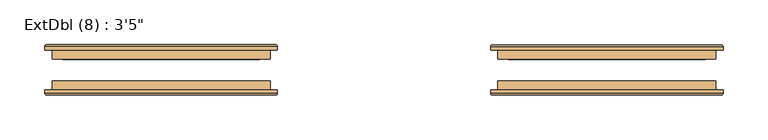
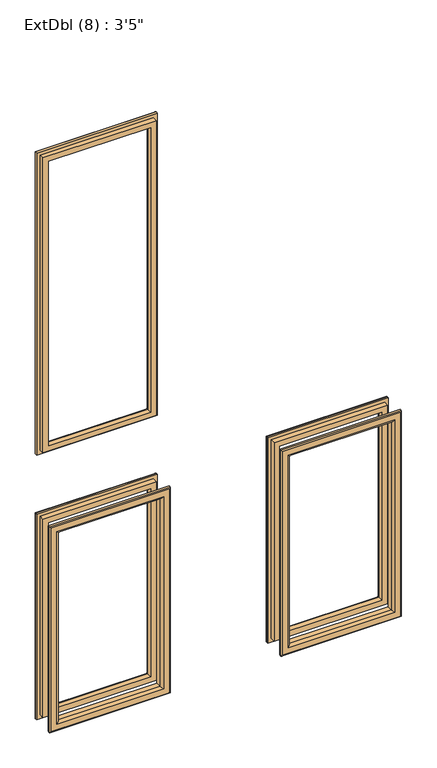
"""IFC4 building model written with IfcOpenShell, lengths in millimetres: door geometry."""

from ifc_helpers import new_model, si_unit, frame, origin, place, context, project, spatial, ellipse_curve, source, transform, mapped, element, save
from ifc_brep_helpers import plane_surface, cylinder_surface, advanced_brep


def door_f6085f53(model_context):
    return source(origin(), model_context, "Body", "AdvancedBrep", [
        advanced_brep(
        [(-377.2, 8.3, 950.5), (-377.2, 4.3, 950.5), (-377.2, 4.3, 1635.3), (-377.2, 8.3, 1635.3), (-375.2, 10.3, 952.5), (-375.2, 10.3, 1633.3), (-357.2, 5.3, 970.5), (-362.2, 10.3, 965.5), (-362.2, 10.3, 1620.3), (-357.2, 5.3, 1615.3), (-357.2, -5.7, 970.5), (-357.2, -5.7, 1615.3), (-369.2, 4.3, 958.5), (-369.2, -5.7, 958.5), (-369.2, -5.7, 1627.3), (-369.2, 4.3, 1627.3), (-118.5, 4.3, 1635.3), (-118.5, 8.3, 1635.3), (-120.5, 10.3, 1633.3), (-133.5, 10.3, 1620.3), (-138.5, 5.3, 1615.3), (-138.5, -5.7, 1615.3), (-126.5, -5.7, 1627.3), (-126.5, 4.3, 1627.3), (-118.5, 4.3, 950.5), (-118.5, 8.3, 950.5), (-120.5, 10.3, 952.5), (-133.5, 10.3, 965.5), (-138.5, 5.3, 970.5), (-138.5, -5.7, 970.5), (-126.5, -5.7, 958.5), (-126.5, 4.3, 958.5)],
        [
            (0, 1),
            (1, 2),
            (2, 3),
            (3, 0),
            (4, 0, ellipse_curve(frame((-375.2, 8.3, 952.5), z_axis=(-0.7071067811865472, 0.0, 0.7071067811865477), x_axis=(-0.7071067811865477, 0.0, -0.7071067811865475)), 2.8284271, 2.0)),
            (3, 5, ellipse_curve(frame((-375.2, 8.3, 1633.3), z_axis=(-0.7071067811865475, 0.0, -0.7071067811865475), x_axis=(0.7071067811865474, 0.0, -0.7071067811865476)), 2.8284271, 2.0)),
            (5, 4),
            (6, 7, ellipse_curve(frame((-362.2, 5.3, 965.5), z_axis=(-0.7071067811865472, 0.0, 0.7071067811865477), x_axis=(-0.7071067811865477, 0.0, -0.7071067811865475)), 7.0710678, 5.0)),
            (7, 8),
            (8, 9, ellipse_curve(frame((-362.2, 5.3, 1620.3), z_axis=(-0.7071067811865475, 0.0, -0.7071067811865475), x_axis=(0.7071067811865474, 0.0, -0.7071067811865476)), 7.0710678, 5.0)),
            (9, 6),
            (10, 6),
            (9, 11),
            (11, 10),
            (12, 13),
            (13, 14),
            (14, 15),
            (15, 12),
            (2, 16),
            (16, 17),
            (17, 3),
            (17, 18, ellipse_curve(frame((-120.5, 8.3, 1633.3), z_axis=(-0.7071067811865475, 0.0, 0.7071067811865476), x_axis=(-0.7071067811865476, 0.0, -0.7071067811865475)), 2.8284271, 2.0)),
            (18, 5),
            (8, 19),
            (19, 20, ellipse_curve(frame((-133.5, 5.3, 1620.3), z_axis=(-0.7071067811865475, 0.0, 0.7071067811865476), x_axis=(-0.7071067811865476, 0.0, -0.7071067811865475)), 7.0710678, 5.0)),
            (20, 9),
            (20, 21),
            (21, 11),
            (14, 22),
            (22, 23),
            (23, 15),
            (16, 24),
            (24, 25),
            (25, 17),
            (25, 26, ellipse_curve(frame((-120.5, 8.3, 952.5), z_axis=(0.7071067811865478, 0.0, 0.7071067811865472), x_axis=(-0.7071067811865472, 0.0, 0.7071067811865478)), 2.8284271, 2.0)),
            (26, 18),
            (19, 27),
            (27, 28, ellipse_curve(frame((-133.5, 5.3, 965.5), z_axis=(0.7071067811865478, 0.0, 0.7071067811865472), x_axis=(-0.7071067811865472, 0.0, 0.7071067811865478)), 7.0710678, 5.0)),
            (28, 20),
            (28, 29),
            (29, 21),
            (22, 30),
            (30, 31),
            (31, 23),
            (24, 1),
            (0, 25),
            (4, 26),
            (7, 27),
            (6, 28),
            (10, 29),
            (13, 30),
            (12, 31),
        ],
        [
            plane_surface(frame((-377.2, 4.3, 950.5), z_axis=(-1.0, 0.0, 0.0), x_axis=(0.0, 0.0, 1.0))),
            cylinder_surface(frame((-375.2, 8.3, 958.5), z_axis=(0.0, 0.0, -1.0), x_axis=(-1.0, 0.0, 0.0)), 2.0),
            cylinder_surface(frame((-362.2, 5.3, 958.5), z_axis=(0.0, 0.0, -1.0), x_axis=(-1.0, 0.0, 0.0)), 5.0),
            plane_surface(frame((-357.2, 5.3, 970.5), z_axis=(1.0, 0.0, 0.0), x_axis=(0.0, 0.0, 1.0))),
            plane_surface(frame((-369.2, -5.7, 958.5), z_axis=(-1.0, 0.0, 0.0), x_axis=(0.0, 0.0, 1.0))),
            plane_surface(frame((-377.2, 4.3, 1635.3), z_axis=(0.0, 0.0, 1.0), x_axis=(1.0, 0.0, 0.0))),
            cylinder_surface(frame((-369.2, 8.3, 1633.3), z_axis=(-1.0, 0.0, 0.0), x_axis=(0.0, 0.0, 1.0)), 2.0),
            cylinder_surface(frame((-369.2, 5.3, 1620.3), z_axis=(-1.0, 0.0, 0.0), x_axis=(0.0, 0.0, 1.0)), 5.0),
            plane_surface(frame((-357.2, 5.3, 1615.3), z_axis=(0.0, 0.0, -1.0), x_axis=(1.0, 0.0, 0.0))),
            plane_surface(frame((-369.2, -5.7, 1627.3), z_axis=(0.0, 0.0, 1.0), x_axis=(1.0, 0.0, 0.0))),
            plane_surface(frame((-118.5, 4.3, 1635.3), z_axis=(1.0, 0.0, 0.0), x_axis=(0.0, 0.0, -1.0))),
            cylinder_surface(frame((-120.5, 8.3, 1627.3), z_axis=(0.0, 0.0, 1.0), x_axis=(1.0, 0.0, 0.0)), 2.0),
            cylinder_surface(frame((-133.5, 5.3, 1627.3), z_axis=(0.0, 0.0, 1.0), x_axis=(1.0, 0.0, 0.0)), 5.0),
            plane_surface(frame((-138.5, 5.3, 1615.3), z_axis=(-1.0, 0.0, 0.0), x_axis=(0.0, 0.0, -1.0))),
            plane_surface(frame((-126.5, -5.7, 1627.3), z_axis=(1.0, 0.0, 0.0), x_axis=(0.0, 0.0, -1.0))),
            plane_surface(frame((-118.5, 4.3, 950.5), z_axis=(0.0, 0.0, -1.0), x_axis=(-1.0, 0.0, 0.0))),
            cylinder_surface(frame((-126.5, 8.3, 952.5), z_axis=(1.0, 0.0, 0.0), x_axis=(0.0, 0.0, -1.0)), 2.0),
            plane_surface(frame((-120.5, 10.3, 952.5), z_axis=(0.0, 1.0, 0.0), x_axis=(-1.0, 0.0, 0.0))),
            cylinder_surface(frame((-126.5, 5.3, 965.5), z_axis=(1.0, 0.0, 0.0), x_axis=(0.0, 0.0, -1.0)), 5.0),
            plane_surface(frame((-138.5, 5.3, 970.5), z_axis=(0.0, 0.0, 1.0), x_axis=(-1.0, 0.0, 0.0))),
            plane_surface(frame((-138.5, -5.7, 970.5), z_axis=(0.0, -1.0, 0.0), x_axis=(-1.0, 0.0, 0.0))),
            plane_surface(frame((-126.5, -5.7, 958.5), z_axis=(0.0, 0.0, -1.0), x_axis=(-1.0, 0.0, 0.0))),
            plane_surface(frame((-126.5, 4.3, 958.5), z_axis=(0.0, -1.0, 0.0), x_axis=(-1.0, 0.0, 0.0))),
        ],
        [
            (0, [[1, 2, 3, 4]]),
            (1, [[5, -4, 6, 7]]),
            (2, [[8, 9, 10, 11]]),
            (3, [[12, -11, 13, 14]]),
            (4, [[15, 16, 17, 18]]),
            (5, [[-3, 19, 20, 21]]),
            (6, [[-6, -21, 22, 23]]),
            (7, [[-10, 24, 25, 26]]),
            (8, [[-13, -26, 27, 28]]),
            (9, [[-17, 29, 30, 31]]),
            (10, [[-20, 32, 33, 34]]),
            (11, [[-22, -34, 35, 36]]),
            (12, [[-25, 37, 38, 39]]),
            (13, [[-27, -39, 40, 41]]),
            (14, [[-30, 42, 43, 44]]),
            (15, [[-33, 45, -1, 46]]),
            (16, [[-35, -46, -5, 47]]),
            (17, [[-23, -36, -47, -7], [48, -37, -24, -9]]),
            (18, [[-38, -48, -8, 49]]),
            (19, [[-40, -49, -12, 50]]),
            (20, [[51, -42, -29, -16], [-28, -41, -50, -14]]),
            (21, [[-43, -51, -15, 52]]),
            (22, [[-45, -32, -19, -2], [-31, -44, -52, -18]]),
        ],
    ),
        advanced_brep(
        [(126.5, -5.7, 808.5), (126.5, 4.3, 808.5), (126.5, 4.3, 358.5), (126.5, -5.7, 358.5), (138.5, 5.3, 796.5), (138.5, -5.7, 796.5), (138.5, -5.7, 370.5), (138.5, 5.3, 370.5), (133.5, 10.3, 801.5), (133.5, 10.3, 365.5), (118.5, 8.3, 816.5), (120.5, 10.3, 814.5), (120.5, 10.3, 352.5), (118.5, 8.3, 350.5), (118.5, 4.3, 816.5), (118.5, 4.3, 350.5), (369.2, 4.3, 358.5), (369.2, -5.7, 358.5), (357.2, -5.7, 370.5), (357.2, 5.3, 370.5), (362.2, 10.3, 365.5), (375.2, 10.3, 352.5), (377.2, 8.3, 350.5), (377.2, 4.3, 350.5), (369.2, 4.3, 808.5), (369.2, -5.7, 808.5), (357.2, -5.7, 796.5), (357.2, 5.3, 796.5), (362.2, 10.3, 801.5), (375.2, 10.3, 814.5), (377.2, 8.3, 816.5), (377.2, 4.3, 816.5)],
        [
            (0, 1),
            (1, 2),
            (2, 3),
            (3, 0),
            (4, 5),
            (5, 6),
            (6, 7),
            (7, 4),
            (8, 4, ellipse_curve(frame((133.5, 5.3, 801.5), z_axis=(-0.7071067811865475, 0.0, -0.7071067811865475), x_axis=(-0.7071067811865474, 0.0, 0.7071067811865476)), 7.0710678, 5.0)),
            (7, 9, ellipse_curve(frame((133.5, 5.3, 365.5), z_axis=(-0.7071067811865475, 0.0, 0.7071067811865475), x_axis=(0.7071067811865474, 0.0, 0.7071067811865476)), 7.0710678, 5.0)),
            (9, 8),
            (10, 11, ellipse_curve(frame((120.5, 8.3, 814.5), z_axis=(-0.7071067811865475, 0.0, -0.7071067811865475), x_axis=(-0.7071067811865474, 0.0, 0.7071067811865476)), 2.8284271, 2.0)),
            (11, 12),
            (12, 13, ellipse_curve(frame((120.5, 8.3, 352.5), z_axis=(-0.7071067811865475, 0.0, 0.7071067811865475), x_axis=(0.7071067811865474, 0.0, 0.7071067811865476)), 2.8284271, 2.0)),
            (13, 10),
            (14, 10),
            (13, 15),
            (15, 14),
            (2, 16),
            (16, 17),
            (17, 3),
            (6, 18),
            (18, 19),
            (19, 7),
            (19, 20, ellipse_curve(frame((362.2, 5.3, 365.5), z_axis=(-0.7071067811865476, 0.0, -0.7071067811865475), x_axis=(-0.7071067811865475, 0.0, 0.7071067811865476)), 7.0710678, 5.0)),
            (20, 9),
            (12, 21),
            (21, 22, ellipse_curve(frame((375.2, 8.3, 352.5), z_axis=(-0.7071067811865476, 0.0, -0.7071067811865475), x_axis=(-0.7071067811865475, 0.0, 0.7071067811865476)), 2.8284271, 2.0)),
            (22, 13),
            (22, 23),
            (23, 15),
            (16, 24),
            (24, 25),
            (25, 17),
            (18, 26),
            (26, 27),
            (27, 19),
            (27, 28, ellipse_curve(frame((362.2, 5.3, 801.5), z_axis=(0.7071067811865475, 0.0, -0.7071067811865476), x_axis=(-0.7071067811865476, 0.0, -0.7071067811865475)), 7.0710678, 5.0)),
            (28, 20),
            (21, 29),
            (29, 30, ellipse_curve(frame((375.2, 8.3, 814.5), z_axis=(0.7071067811865475, 0.0, -0.7071067811865476), x_axis=(-0.7071067811865476, 0.0, -0.7071067811865475)), 2.8284271, 2.0)),
            (30, 22),
            (30, 31),
            (31, 23),
            (31, 14),
            (1, 24),
            (0, 25),
            (5, 26),
            (4, 27),
            (8, 28),
            (11, 29),
            (10, 30),
        ],
        [
            plane_surface(frame((126.5, 4.3, 808.5), z_axis=(-1.0, 0.0, 0.0), x_axis=(0.0, 0.0, -1.0))),
            plane_surface(frame((138.5, -5.7, 796.5), z_axis=(1.0, 0.0, 0.0), x_axis=(0.0, 0.0, -1.0))),
            cylinder_surface(frame((133.5, 5.3, 808.5), z_axis=(0.0, 0.0, 1.0), x_axis=(-1.0, 0.0, 0.0)), 5.0),
            cylinder_surface(frame((120.5, 8.3, 808.5), z_axis=(0.0, 0.0, 1.0), x_axis=(-1.0, 0.0, 0.0)), 2.0),
            plane_surface(frame((118.5, 8.3, 816.5), z_axis=(-1.0, 0.0, 0.0), x_axis=(0.0, 0.0, -1.0))),
            plane_surface(frame((126.5, 4.3, 358.5), z_axis=(0.0, 0.0, -1.0), x_axis=(1.0, 0.0, 0.0))),
            plane_surface(frame((138.5, -5.7, 370.5), z_axis=(0.0, 0.0, 1.0), x_axis=(1.0, 0.0, 0.0))),
            cylinder_surface(frame((126.5, 5.3, 365.5), z_axis=(-1.0, 0.0, 0.0), x_axis=(0.0, 0.0, -1.0)), 5.0),
            cylinder_surface(frame((126.5, 8.3, 352.5), z_axis=(-1.0, 0.0, 0.0), x_axis=(0.0, 0.0, -1.0)), 2.0),
            plane_surface(frame((118.5, 8.3, 350.5), z_axis=(0.0, 0.0, -1.0), x_axis=(1.0, 0.0, 0.0))),
            plane_surface(frame((369.2, 4.3, 358.5), z_axis=(1.0, 0.0, 0.0), x_axis=(0.0, 0.0, 1.0))),
            plane_surface(frame((357.2, -5.7, 370.5), z_axis=(-1.0, 0.0, 0.0), x_axis=(0.0, 0.0, 1.0))),
            cylinder_surface(frame((362.2, 5.3, 358.5), z_axis=(0.0, 0.0, -1.0), x_axis=(1.0, 0.0, 0.0)), 5.0),
            cylinder_surface(frame((375.2, 8.3, 358.5), z_axis=(0.0, 0.0, -1.0), x_axis=(1.0, 0.0, 0.0)), 2.0),
            plane_surface(frame((377.2, 8.3, 350.5), z_axis=(1.0, 0.0, 0.0), x_axis=(0.0, 0.0, 1.0))),
            plane_surface(frame((377.2, 4.3, 816.5), z_axis=(0.0, -1.0, 0.0), x_axis=(-1.0, 0.0, 0.0))),
            plane_surface(frame((369.2, 4.3, 808.5), z_axis=(0.0, 0.0, 1.0), x_axis=(-1.0, 0.0, 0.0))),
            plane_surface(frame((369.2, -5.7, 808.5), z_axis=(0.0, -1.0, 0.0), x_axis=(-1.0, 0.0, 0.0))),
            plane_surface(frame((357.2, -5.7, 796.5), z_axis=(0.0, 0.0, -1.0), x_axis=(-1.0, 0.0, 0.0))),
            cylinder_surface(frame((369.2, 5.3, 801.5), z_axis=(1.0, 0.0, 0.0), x_axis=(0.0, 0.0, 1.0)), 5.0),
            plane_surface(frame((362.2, 10.3, 801.5), z_axis=(0.0, 1.0, 0.0), x_axis=(-1.0, 0.0, 0.0))),
            cylinder_surface(frame((369.2, 8.3, 814.5), z_axis=(1.0, 0.0, 0.0), x_axis=(0.0, 0.0, 1.0)), 2.0),
            plane_surface(frame((377.2, 8.3, 816.5), z_axis=(0.0, 0.0, 1.0), x_axis=(-1.0, 0.0, 0.0))),
        ],
        [
            (0, [[1, 2, 3, 4]]),
            (1, [[5, 6, 7, 8]]),
            (2, [[9, -8, 10, 11]]),
            (3, [[12, 13, 14, 15]]),
            (4, [[16, -15, 17, 18]]),
            (5, [[-3, 19, 20, 21]]),
            (6, [[-7, 22, 23, 24]]),
            (7, [[-10, -24, 25, 26]]),
            (8, [[-14, 27, 28, 29]]),
            (9, [[-17, -29, 30, 31]]),
            (10, [[-20, 32, 33, 34]]),
            (11, [[-23, 35, 36, 37]]),
            (12, [[-25, -37, 38, 39]]),
            (13, [[-28, 40, 41, 42]]),
            (14, [[-30, -42, 43, 44]]),
            (15, [[-31, -44, 45, -18], [46, -32, -19, -2]]),
            (16, [[-33, -46, -1, 47]]),
            (17, [[-21, -34, -47, -4], [48, -35, -22, -6]]),
            (18, [[-36, -48, -5, 49]]),
            (19, [[-38, -49, -9, 50]]),
            (20, [[51, -40, -27, -13], [-26, -39, -50, -11]]),
            (21, [[-41, -51, -12, 52]]),
            (22, [[-43, -52, -16, -45]]),
        ],
    ),
        advanced_brep(
        [(369.2, -29.7, 808.5), (369.2, -39.7, 808.5), (369.2, -39.7, 358.5), (369.2, -29.7, 358.5), (357.2, -40.7, 796.5), (357.2, -29.7, 796.5), (357.2, -29.7, 370.5), (357.2, -40.7, 370.5), (362.2, -45.7, 801.5), (362.2, -45.7, 365.5), (377.2, -43.7, 816.5), (375.2, -45.7, 814.5), (375.2, -45.7, 352.5), (377.2, -43.7, 350.5), (377.2, -39.7, 816.5), (377.2, -39.7, 350.5), (126.5, -39.7, 358.5), (126.5, -29.7, 358.5), (138.5, -29.7, 370.5), (138.5, -40.7, 370.5), (133.5, -45.7, 365.5), (120.5, -45.7, 352.5), (118.5, -43.7, 350.5), (118.5, -39.7, 350.5), (126.5, -39.7, 808.5), (126.5, -29.7, 808.5), (138.5, -29.7, 796.5), (138.5, -40.7, 796.5), (133.5, -45.7, 801.5), (120.5, -45.7, 814.5), (118.5, -43.7, 816.5), (118.5, -39.7, 816.5)],
        [
            (0, 1),
            (1, 2),
            (2, 3),
            (3, 0),
            (4, 5),
            (5, 6),
            (6, 7),
            (7, 4),
            (8, 4, ellipse_curve(frame((362.2, -40.7, 801.5), z_axis=(0.7071067811865519, 0.0, -0.707106781186543), x_axis=(0.7071067811865429, 0.0, 0.7071067811865521)), 7.0710678, 5.0)),
            (7, 9, ellipse_curve(frame((362.2, -40.7, 365.5), z_axis=(0.7071067811865429, 0.0, 0.707106781186552), x_axis=(-0.7071067811865519, 0.0, 0.707106781186543)), 7.0710678, 5.0)),
            (9, 8),
            (10, 11, ellipse_curve(frame((375.2, -43.7, 814.5), z_axis=(0.7071067811865519, 0.0, -0.707106781186543), x_axis=(0.7071067811865429, 0.0, 0.7071067811865521)), 2.8284271, 2.0)),
            (11, 12),
            (12, 13, ellipse_curve(frame((375.2, -43.7, 352.5), z_axis=(0.7071067811865429, 0.0, 0.707106781186552), x_axis=(-0.7071067811865519, 0.0, 0.707106781186543)), 2.8284271, 2.0)),
            (13, 10),
            (14, 10),
            (13, 15),
            (15, 14),
            (2, 16),
            (16, 17),
            (17, 3),
            (6, 18),
            (18, 19),
            (19, 7),
            (19, 20, ellipse_curve(frame((133.5, -40.7, 365.5), z_axis=(0.707106781186552, 0.0, -0.7071067811865429), x_axis=(0.707106781186543, 0.0, 0.7071067811865519)), 7.0710678, 5.0)),
            (20, 9),
            (12, 21),
            (21, 22, ellipse_curve(frame((120.5, -43.7, 352.5), z_axis=(0.707106781186552, 0.0, -0.7071067811865429), x_axis=(0.707106781186543, 0.0, 0.7071067811865519)), 2.8284271, 2.0)),
            (22, 13),
            (22, 23),
            (23, 15),
            (16, 24),
            (24, 25),
            (25, 17),
            (18, 26),
            (26, 27),
            (27, 19),
            (27, 28, ellipse_curve(frame((133.5, -40.7, 801.5), z_axis=(-0.7071067811865431, 0.0, -0.707106781186552), x_axis=(0.7071067811865521, 0.0, -0.7071067811865429)), 7.0710678, 5.0)),
            (28, 20),
            (21, 29),
            (29, 30, ellipse_curve(frame((120.5, -43.7, 814.5), z_axis=(-0.7071067811865431, 0.0, -0.707106781186552), x_axis=(0.7071067811865521, 0.0, -0.7071067811865429)), 2.8284271, 2.0)),
            (30, 22),
            (30, 31),
            (31, 23),
            (31, 14),
            (1, 24),
            (0, 25),
            (5, 26),
            (4, 27),
            (8, 28),
            (11, 29),
            (10, 30),
        ],
        [
            plane_surface(frame((369.2, -39.7, 808.5), z_axis=(1.0, 0.0, 0.0), x_axis=(0.0, 0.0, -1.0))),
            plane_surface(frame((357.2, -29.7, 796.5), z_axis=(-1.0, 0.0, 0.0), x_axis=(0.0, 0.0, -1.0))),
            cylinder_surface(frame((362.2, -40.7, 808.5), z_axis=(0.0, 0.0, 1.0), x_axis=(1.0, 0.0, 0.0)), 5.0),
            cylinder_surface(frame((375.2, -43.7, 808.5), z_axis=(0.0, 0.0, 1.0), x_axis=(1.0, 0.0, 0.0)), 2.0),
            plane_surface(frame((377.2, -43.7, 816.5), z_axis=(1.0, 0.0, 0.0), x_axis=(0.0, 0.0, -1.0))),
            plane_surface(frame((369.2, -39.7, 358.5), z_axis=(0.0, 0.0, -1.0), x_axis=(-1.0, 0.0, 0.0))),
            plane_surface(frame((357.2, -29.7, 370.5), z_axis=(0.0, 0.0, 1.0), x_axis=(-1.0, 0.0, 0.0))),
            cylinder_surface(frame((369.2, -40.7, 365.5), z_axis=(1.0, 0.0, 0.0), x_axis=(0.0, 0.0, -1.0)), 5.0),
            cylinder_surface(frame((369.2, -43.7, 352.5), z_axis=(1.0, 0.0, 0.0), x_axis=(0.0, 0.0, -1.0)), 2.0),
            plane_surface(frame((377.2, -43.7, 350.5), z_axis=(0.0, 0.0, -1.0), x_axis=(-1.0, 0.0, 0.0))),
            plane_surface(frame((126.5, -39.7, 358.5), z_axis=(-1.0, 0.0, 0.0), x_axis=(0.0, 0.0, 1.0))),
            plane_surface(frame((138.5, -29.7, 370.5), z_axis=(1.0, 0.0, 0.0), x_axis=(0.0, 0.0, 1.0))),
            cylinder_surface(frame((133.5, -40.7, 358.5), z_axis=(0.0, 0.0, -1.0), x_axis=(-1.0, 0.0, 0.0)), 5.0),
            cylinder_surface(frame((120.5, -43.7, 358.5), z_axis=(0.0, 0.0, -1.0), x_axis=(-1.0, 0.0, 0.0)), 2.0),
            plane_surface(frame((118.5, -43.7, 350.5), z_axis=(-1.0, 0.0, 0.0), x_axis=(0.0, 0.0, 1.0))),
            plane_surface(frame((118.5, -39.7, 816.5), z_axis=(0.0, 1.0, 0.0), x_axis=(1.0, 0.0, 0.0))),
            plane_surface(frame((126.5, -39.7, 808.5), z_axis=(0.0, 0.0, 1.0), x_axis=(1.0, 0.0, 0.0))),
            plane_surface(frame((126.5, -29.7, 808.5), z_axis=(0.0, 1.0, 0.0), x_axis=(1.0, 0.0, 0.0))),
            plane_surface(frame((138.5, -29.7, 796.5), z_axis=(0.0, 0.0, -1.0), x_axis=(1.0, 0.0, 0.0))),
            cylinder_surface(frame((126.5, -40.7, 801.5), z_axis=(-1.0, 0.0, 0.0), x_axis=(0.0, 0.0, 1.0)), 5.0),
            plane_surface(frame((133.5, -45.7, 801.5), z_axis=(0.0, -1.0, 0.0), x_axis=(1.0, 0.0, 0.0))),
            cylinder_surface(frame((126.5, -43.7, 814.5), z_axis=(-1.0, 0.0, 0.0), x_axis=(0.0, 0.0, 1.0)), 2.0),
            plane_surface(frame((118.5, -43.7, 816.5), z_axis=(0.0, 0.0, 1.0), x_axis=(1.0, 0.0, 0.0))),
        ],
        [
            (0, [[1, 2, 3, 4]]),
            (1, [[5, 6, 7, 8]]),
            (2, [[9, -8, 10, 11]]),
            (3, [[12, 13, 14, 15]]),
            (4, [[16, -15, 17, 18]]),
            (5, [[-3, 19, 20, 21]]),
            (6, [[-7, 22, 23, 24]]),
            (7, [[-10, -24, 25, 26]]),
            (8, [[-14, 27, 28, 29]]),
            (9, [[-17, -29, 30, 31]]),
            (10, [[-20, 32, 33, 34]]),
            (11, [[-23, 35, 36, 37]]),
            (12, [[-25, -37, 38, 39]]),
            (13, [[-28, 40, 41, 42]]),
            (14, [[-30, -42, 43, 44]]),
            (15, [[-31, -44, 45, -18], [46, -32, -19, -2]]),
            (16, [[-33, -46, -1, 47]]),
            (17, [[-21, -34, -47, -4], [48, -35, -22, -6]]),
            (18, [[-36, -48, -5, 49]]),
            (19, [[-38, -49, -9, 50]]),
            (20, [[51, -40, -27, -13], [-26, -39, -50, -11]]),
            (21, [[-41, -51, -12, 52]]),
            (22, [[-43, -52, -16, -45]]),
        ],
    ),
        advanced_brep(
        [(-369.2, -5.7, 808.5), (-369.2, 4.3, 808.5), (-369.2, 4.3, 358.5), (-369.2, -5.7, 358.5), (-357.2, 5.3, 796.5), (-357.2, -5.7, 796.5), (-357.2, -5.7, 370.5), (-357.2, 5.3, 370.5), (-362.2, 10.3, 801.5), (-362.2, 10.3, 365.5), (-377.2, 8.3, 816.5), (-375.2, 10.3, 814.5), (-375.2, 10.3, 352.5), (-377.2, 8.3, 350.5), (-377.2, 4.3, 816.5), (-377.2, 4.3, 350.5), (-126.5, 4.3, 358.5), (-126.5, -5.7, 358.5), (-138.5, -5.7, 370.5), (-138.5, 5.3, 370.5), (-133.5, 10.3, 365.5), (-120.5, 10.3, 352.5), (-118.5, 8.3, 350.5), (-118.5, 4.3, 350.5), (-126.5, 4.3, 808.5), (-126.5, -5.7, 808.5), (-138.5, -5.7, 796.5), (-138.5, 5.3, 796.5), (-133.5, 10.3, 801.5), (-120.5, 10.3, 814.5), (-118.5, 8.3, 816.5), (-118.5, 4.3, 816.5)],
        [
            (0, 1),
            (1, 2),
            (2, 3),
            (3, 0),
            (4, 5),
            (5, 6),
            (6, 7),
            (7, 4),
            (8, 4, ellipse_curve(frame((-362.2, 5.3, 801.5), z_axis=(-0.7071067811865478, 0.0, -0.7071067811865474), x_axis=(-0.7071067811865474, 0.0, 0.7071067811865476)), 7.0710678, 5.0)),
            (7, 9, ellipse_curve(frame((-362.2, 5.3, 365.5), z_axis=(-0.7071067811865475, 0.0, 0.7071067811865475), x_axis=(0.7071067811865474, 0.0, 0.7071067811865476)), 7.0710678, 5.0)),
            (9, 8),
            (10, 11, ellipse_curve(frame((-375.2, 8.3, 814.5), z_axis=(-0.7071067811865478, 0.0, -0.7071067811865474), x_axis=(-0.7071067811865474, 0.0, 0.7071067811865476)), 2.8284271, 2.0)),
            (11, 12),
            (12, 13, ellipse_curve(frame((-375.2, 8.3, 352.5), z_axis=(-0.7071067811865475, 0.0, 0.7071067811865475), x_axis=(0.7071067811865474, 0.0, 0.7071067811865476)), 2.8284271, 2.0)),
            (13, 10),
            (14, 10),
            (13, 15),
            (15, 14),
            (2, 16),
            (16, 17),
            (17, 3),
            (6, 18),
            (18, 19),
            (19, 7),
            (19, 20, ellipse_curve(frame((-133.5, 5.3, 365.5), z_axis=(-0.7071067811865475, 0.0, -0.7071067811865475), x_axis=(-0.7071067811865476, 0.0, 0.7071067811865474)), 7.0710678, 5.0)),
            (20, 9),
            (12, 21),
            (21, 22, ellipse_curve(frame((-120.5, 8.3, 352.5), z_axis=(-0.7071067811865475, 0.0, -0.7071067811865475), x_axis=(-0.7071067811865476, 0.0, 0.7071067811865474)), 2.8284271, 2.0)),
            (22, 13),
            (22, 23),
            (23, 15),
            (16, 24),
            (24, 25),
            (25, 17),
            (18, 26),
            (26, 27),
            (27, 19),
            (27, 28, ellipse_curve(frame((-133.5, 5.3, 801.5), z_axis=(0.7071067811865472, 0.0, -0.7071067811865477), x_axis=(-0.7071067811865477, 0.0, -0.7071067811865475)), 7.0710678, 5.0)),
            (28, 20),
            (21, 29),
            (29, 30, ellipse_curve(frame((-120.5, 8.3, 814.5), z_axis=(0.7071067811865472, 0.0, -0.7071067811865477), x_axis=(-0.7071067811865477, 0.0, -0.7071067811865475)), 2.8284271, 2.0)),
            (30, 22),
            (30, 31),
            (31, 23),
            (31, 14),
            (1, 24),
            (0, 25),
            (5, 26),
            (4, 27),
            (8, 28),
            (11, 29),
            (10, 30),
        ],
        [
            plane_surface(frame((-369.2, 4.3, 808.5), z_axis=(-1.0, 0.0, 0.0), x_axis=(0.0, 0.0, -1.0))),
            plane_surface(frame((-357.2, -5.7, 796.5), z_axis=(1.0, 0.0, 0.0), x_axis=(0.0, 0.0, -1.0))),
            cylinder_surface(frame((-362.2, 5.3, 808.5), z_axis=(0.0, 0.0, 1.0), x_axis=(-1.0, 0.0, 0.0)), 5.0),
            cylinder_surface(frame((-375.2, 8.3, 808.5), z_axis=(0.0, 0.0, 1.0), x_axis=(-1.0, 0.0, 0.0)), 2.0),
            plane_surface(frame((-377.2, 8.3, 816.5), z_axis=(-1.0, 0.0, 0.0), x_axis=(0.0, 0.0, -1.0))),
            plane_surface(frame((-369.2, 4.3, 358.5), z_axis=(0.0, 0.0, -1.0), x_axis=(1.0, 0.0, 0.0))),
            plane_surface(frame((-357.2, -5.7, 370.5), z_axis=(0.0, 0.0, 1.0), x_axis=(1.0, 0.0, 0.0))),
            cylinder_surface(frame((-369.2, 5.3, 365.5), z_axis=(-1.0, 0.0, 0.0), x_axis=(0.0, 0.0, -1.0)), 5.0),
            cylinder_surface(frame((-369.2, 8.3, 352.5), z_axis=(-1.0, 0.0, 0.0), x_axis=(0.0, 0.0, -1.0)), 2.0),
            plane_surface(frame((-377.2, 8.3, 350.5), z_axis=(0.0, 0.0, -1.0), x_axis=(1.0, 0.0, 0.0))),
            plane_surface(frame((-126.5, 4.3, 358.5), z_axis=(1.0, 0.0, 0.0), x_axis=(0.0, 0.0, 1.0))),
            plane_surface(frame((-138.5, -5.7, 370.5), z_axis=(-1.0, 0.0, 0.0), x_axis=(0.0, 0.0, 1.0))),
            cylinder_surface(frame((-133.5, 5.3, 358.5), z_axis=(0.0, 0.0, -1.0), x_axis=(1.0, 0.0, 0.0)), 5.0),
            cylinder_surface(frame((-120.5, 8.3, 358.5), z_axis=(0.0, 0.0, -1.0), x_axis=(1.0, 0.0, 0.0)), 2.0),
            plane_surface(frame((-118.5, 8.3, 350.5), z_axis=(1.0, 0.0, 0.0), x_axis=(0.0, 0.0, 1.0))),
            plane_surface(frame((-118.5, 4.3, 816.5), z_axis=(0.0, -1.0, 0.0), x_axis=(-1.0, 0.0, 0.0))),
            plane_surface(frame((-126.5, 4.3, 808.5), z_axis=(0.0, 0.0, 1.0), x_axis=(-1.0, 0.0, 0.0))),
            plane_surface(frame((-126.5, -5.7, 808.5), z_axis=(0.0, -1.0, 0.0), x_axis=(-1.0, 0.0, 0.0))),
            plane_surface(frame((-138.5, -5.7, 796.5), z_axis=(0.0, 0.0, -1.0), x_axis=(-1.0, 0.0, 0.0))),
            cylinder_surface(frame((-126.5, 5.3, 801.5), z_axis=(1.0, 0.0, 0.0), x_axis=(0.0, 0.0, 1.0)), 5.0),
            plane_surface(frame((-133.5, 10.3, 801.5), z_axis=(0.0, 1.0, 0.0), x_axis=(-1.0, 0.0, 0.0))),
            cylinder_surface(frame((-126.5, 8.3, 814.5), z_axis=(1.0, 0.0, 0.0), x_axis=(0.0, 0.0, 1.0)), 2.0),
            plane_surface(frame((-118.5, 8.3, 816.5), z_axis=(0.0, 0.0, 1.0), x_axis=(-1.0, 0.0, 0.0))),
        ],
        [
            (0, [[1, 2, 3, 4]]),
            (1, [[5, 6, 7, 8]]),
            (2, [[9, -8, 10, 11]]),
            (3, [[12, 13, 14, 15]]),
            (4, [[16, -15, 17, 18]]),
            (5, [[-3, 19, 20, 21]]),
            (6, [[-7, 22, 23, 24]]),
            (7, [[-10, -24, 25, 26]]),
            (8, [[-14, 27, 28, 29]]),
            (9, [[-17, -29, 30, 31]]),
            (10, [[-20, 32, 33, 34]]),
            (11, [[-23, 35, 36, 37]]),
            (12, [[-25, -37, 38, 39]]),
            (13, [[-28, 40, 41, 42]]),
            (14, [[-30, -42, 43, 44]]),
            (15, [[-31, -44, 45, -18], [46, -32, -19, -2]]),
            (16, [[-33, -46, -1, 47]]),
            (17, [[-21, -34, -47, -4], [48, -35, -22, -6]]),
            (18, [[-36, -48, -5, 49]]),
            (19, [[-38, -49, -9, 50]]),
            (20, [[51, -40, -27, -13], [-26, -39, -50, -11]]),
            (21, [[-41, -51, -12, 52]]),
            (22, [[-43, -52, -16, -45]]),
        ],
    ),
        advanced_brep(
        [(-126.5, -29.7, 808.5), (-126.5, -39.7, 808.5), (-126.5, -39.7, 358.5), (-126.5, -29.7, 358.5), (-138.5, -40.7, 796.5), (-138.5, -29.7, 796.5), (-138.5, -29.7, 370.5), (-138.5, -40.7, 370.5), (-133.5, -45.7, 801.5), (-133.5, -45.7, 365.5), (-118.5, -43.7, 816.5), (-120.5, -45.7, 814.5), (-120.5, -45.7, 352.5), (-118.5, -43.7, 350.5), (-118.5, -39.7, 816.5), (-118.5, -39.7, 350.5), (-369.2, -39.7, 358.5), (-369.2, -29.7, 358.5), (-357.2, -29.7, 370.5), (-357.2, -40.7, 370.5), (-362.2, -45.7, 365.5), (-375.2, -45.7, 352.5), (-377.2, -43.7, 350.5), (-377.2, -39.7, 350.5), (-369.2, -39.7, 808.5), (-369.2, -29.7, 808.5), (-357.2, -29.7, 796.5), (-357.2, -40.7, 796.5), (-362.2, -45.7, 801.5), (-375.2, -45.7, 814.5), (-377.2, -43.7, 816.5), (-377.2, -39.7, 816.5)],
        [
            (0, 1),
            (1, 2),
            (2, 3),
            (3, 0),
            (4, 5),
            (5, 6),
            (6, 7),
            (7, 4),
            (8, 4, ellipse_curve(frame((-133.5, -40.7, 801.5), z_axis=(0.7071067811865521, 0.0, -0.707106781186543), x_axis=(0.707106781186543, 0.0, 0.707106781186552)), 7.0710678, 5.0)),
            (7, 9, ellipse_curve(frame((-133.5, -40.7, 365.5), z_axis=(0.707106781186543, 0.0, 0.707106781186552), x_axis=(-0.707106781186552, 0.0, 0.707106781186543)), 7.0710678, 5.0)),
            (9, 8),
            (10, 11, ellipse_curve(frame((-120.5, -43.7, 814.5), z_axis=(0.7071067811865521, 0.0, -0.707106781186543), x_axis=(0.707106781186543, 0.0, 0.707106781186552)), 2.8284271, 2.0)),
            (11, 12),
            (12, 13, ellipse_curve(frame((-120.5, -43.7, 352.5), z_axis=(0.707106781186543, 0.0, 0.707106781186552), x_axis=(-0.707106781186552, 0.0, 0.707106781186543)), 2.8284271, 2.0)),
            (13, 10),
            (14, 10),
            (13, 15),
            (15, 14),
            (2, 16),
            (16, 17),
            (17, 3),
            (6, 18),
            (18, 19),
            (19, 7),
            (19, 20, ellipse_curve(frame((-362.2, -40.7, 365.5), z_axis=(0.707106781186552, 0.0, -0.7071067811865429), x_axis=(0.707106781186543, 0.0, 0.707106781186552)), 7.0710678, 5.0)),
            (20, 9),
            (12, 21),
            (21, 22, ellipse_curve(frame((-375.2, -43.7, 352.5), z_axis=(0.707106781186552, 0.0, -0.7071067811865429), x_axis=(0.707106781186543, 0.0, 0.707106781186552)), 2.8284271, 2.0)),
            (22, 13),
            (22, 23),
            (23, 15),
            (16, 24),
            (24, 25),
            (25, 17),
            (18, 26),
            (26, 27),
            (27, 19),
            (27, 28, ellipse_curve(frame((-362.2, -40.7, 801.5), z_axis=(-0.7071067811865428, 0.0, -0.7071067811865521), x_axis=(0.707106781186552, 0.0, -0.7071067811865429)), 7.0710678, 5.0)),
            (28, 20),
            (21, 29),
            (29, 30, ellipse_curve(frame((-375.2, -43.7, 814.5), z_axis=(-0.7071067811865428, 0.0, -0.7071067811865521), x_axis=(0.707106781186552, 0.0, -0.7071067811865429)), 2.8284271, 2.0)),
            (30, 22),
            (30, 31),
            (31, 23),
            (31, 14),
            (1, 24),
            (0, 25),
            (5, 26),
            (4, 27),
            (8, 28),
            (11, 29),
            (10, 30),
        ],
        [
            plane_surface(frame((-126.5, -39.7, 808.5), z_axis=(1.0, 0.0, 0.0), x_axis=(0.0, 0.0, -1.0))),
            plane_surface(frame((-138.5, -29.7, 796.5), z_axis=(-1.0, 0.0, 0.0), x_axis=(0.0, 0.0, -1.0))),
            cylinder_surface(frame((-133.5, -40.7, 808.5), z_axis=(0.0, 0.0, 1.0), x_axis=(1.0, 0.0, 0.0)), 5.0),
            cylinder_surface(frame((-120.5, -43.7, 808.5), z_axis=(0.0, 0.0, 1.0), x_axis=(1.0, 0.0, 0.0)), 2.0),
            plane_surface(frame((-118.5, -43.7, 816.5), z_axis=(1.0, 0.0, 0.0), x_axis=(0.0, 0.0, -1.0))),
            plane_surface(frame((-126.5, -39.7, 358.5), z_axis=(0.0, 0.0, -1.0), x_axis=(-1.0, 0.0, 0.0))),
            plane_surface(frame((-138.5, -29.7, 370.5), z_axis=(0.0, 0.0, 1.0), x_axis=(-1.0, 0.0, 0.0))),
            cylinder_surface(frame((-126.5, -40.7, 365.5), z_axis=(1.0, 0.0, 0.0), x_axis=(0.0, 0.0, -1.0)), 5.0),
            cylinder_surface(frame((-126.5, -43.7, 352.5), z_axis=(1.0, 0.0, 0.0), x_axis=(0.0, 0.0, -1.0)), 2.0),
            plane_surface(frame((-118.5, -43.7, 350.5), z_axis=(0.0, 0.0, -1.0), x_axis=(-1.0, 0.0, 0.0))),
            plane_surface(frame((-369.2, -39.7, 358.5), z_axis=(-1.0, 0.0, 0.0), x_axis=(0.0, 0.0, 1.0))),
            plane_surface(frame((-357.2, -29.7, 370.5), z_axis=(1.0, 0.0, 0.0), x_axis=(0.0, 0.0, 1.0))),
            cylinder_surface(frame((-362.2, -40.7, 358.5), z_axis=(0.0, 0.0, -1.0), x_axis=(-1.0, 0.0, 0.0)), 5.0),
            cylinder_surface(frame((-375.2, -43.7, 358.5), z_axis=(0.0, 0.0, -1.0), x_axis=(-1.0, 0.0, 0.0)), 2.0),
            plane_surface(frame((-377.2, -43.7, 350.5), z_axis=(-1.0, 0.0, 0.0), x_axis=(0.0, 0.0, 1.0))),
            plane_surface(frame((-377.2, -39.7, 816.5), z_axis=(0.0, 1.0, 0.0), x_axis=(1.0, 0.0, 0.0))),
            plane_surface(frame((-369.2, -39.7, 808.5), z_axis=(0.0, 0.0, 1.0), x_axis=(1.0, 0.0, 0.0))),
            plane_surface(frame((-369.2, -29.7, 808.5), z_axis=(0.0, 1.0, 0.0), x_axis=(1.0, 0.0, 0.0))),
            plane_surface(frame((-357.2, -29.7, 796.5), z_axis=(0.0, 0.0, -1.0), x_axis=(1.0, 0.0, 0.0))),
            cylinder_surface(frame((-369.2, -40.7, 801.5), z_axis=(-1.0, 0.0, 0.0), x_axis=(0.0, 0.0, 1.0)), 5.0),
            plane_surface(frame((-362.2, -45.7, 801.5), z_axis=(0.0, -1.0, 0.0), x_axis=(1.0, 0.0, 0.0))),
            cylinder_surface(frame((-369.2, -43.7, 814.5), z_axis=(-1.0, 0.0, 0.0), x_axis=(0.0, 0.0, 1.0)), 2.0),
            plane_surface(frame((-377.2, -43.7, 816.5), z_axis=(0.0, 0.0, 1.0), x_axis=(1.0, 0.0, 0.0))),
        ],
        [
            (0, [[1, 2, 3, 4]]),
            (1, [[5, 6, 7, 8]]),
            (2, [[9, -8, 10, 11]]),
            (3, [[12, 13, 14, 15]]),
            (4, [[16, -15, 17, 18]]),
            (5, [[-3, 19, 20, 21]]),
            (6, [[-7, 22, 23, 24]]),
            (7, [[-10, -24, 25, 26]]),
            (8, [[-14, 27, 28, 29]]),
            (9, [[-17, -29, 30, 31]]),
            (10, [[-20, 32, 33, 34]]),
            (11, [[-23, 35, 36, 37]]),
            (12, [[-25, -37, 38, 39]]),
            (13, [[-28, 40, 41, 42]]),
            (14, [[-30, -42, 43, 44]]),
            (15, [[-31, -44, 45, -18], [46, -32, -19, -2]]),
            (16, [[-33, -46, -1, 47]]),
            (17, [[-21, -34, -47, -4], [48, -35, -22, -6]]),
            (18, [[-36, -48, -5, 49]]),
            (19, [[-38, -49, -9, 50]]),
            (20, [[51, -40, -27, -13], [-26, -39, -50, -11]]),
            (21, [[-41, -51, -12, 52]]),
            (22, [[-43, -52, -16, -45]]),
        ],
    ),
    ])


if __name__ == "__main__":
    model = new_model("IFC4")
    model_context = context("Model", 3, world=origin())
    ifc_project = project(units=[si_unit("LENGTHUNIT", "METRE", prefix="MILLI")], contexts=[model_context])
    site = spatial("IfcSite", under=ifc_project)
    building = spatial("IfcBuilding", under=site)
    placement = place(None, origin())
    door_shape = door_f6085f53(model_context)
    element("IfcDoor", 1, ObjectType="ExtDbl (8) : 3'5\"", at=placement, inside=building, context=model_context, shape_type="MappedRepresentation", body=[
        mapped(door_shape, transform((0.0, 0.0, 0.0), x_axis=(1.0, 0.0, 0.0), y_axis=(0.0, 1.0, 0.0), z_axis=(0.0, 0.0, 1.0))),
    ])
    save(model, "model.ifc")

# Revit data of these elements
# Type "ExtDbl (8) : 3'5\""
#   Type Mark = "46"
#   Operation = "DoubleDoorSingleSwing"
#   Keynote = "L20"
#   Wrap Layers (Int) from Ext = 0' - 6.98819"
#   Wrap Layers (Ext) from Ext = 0' - 4.03543"
#   Top of Lock Rail = 2' - 11.43307"
#   Thickness = 0' - 1.73228"
#   Stile Shutting = 0' - 4.92126"
#   Stile - Top Rail = 0' - 5.90551"
#   Stile - Lock Rail = 0' - 5.90551"
#   Stile - Hanging = 0' - 3.93701"
#   Stile - Bottom Rail = 0' - 11.81102"
#   Rough Width = 3' - 5"
#   Rough Height = 6' - 0"
#   O/A Frame Width = 0' - 2.51969"
#   Handle Z Distance = 3' - 1.40157"
#   Glazing Thickness = 0' - 0.94488"
#   FrameWidth = 0' - 1.65354"
#   FrameOffset - External = 0' - 2.55906"
#   FrameDepth = 0' - 3.50394"
#   Door Panel Width = 1' - 6.41339"
#   Door Panel Thickness = 0' - 1.73228"
#   Door Panel Height = 5' - 7.66929"
#   Cill Thickness = 0' - 2.14567"
#   Cill Projection = 0' - 1.1811"
#   Handle X Distance = 0' - 2.95276"
#   Height = 6' - 0"
#   Structural Tolerance = 0' - 0.25591"
#   Tolerance = 0' - 0.11811"
#   Undercut = 0' - 0.15748"
#   Width = 3' - 5"
#   Cill Extension = 0' - 0.98425"
#   Cavity Closer Width = 0' - 1.9685"
#   Cavity Closer Offset from Ext = 0' - 4.03543"
#   Cavity Closer Depth = 0' - 3.34646"
#   Vis - Ironmongery = yes
#   Vis - Cavity Closers = yes
#   Function = 1
#   Material Glass = Door - Glazing
#   Handle Style = element 367520
#   Material Door = Door - Panel
#   Material Ironmongery = Door - Handle
#   Wall Closure = (empty or 0)
# Element 1 (IfcDoor, "ExtDbl (8) : 3'5\"")
#   Materials on its faces: "Door - Panel", "Door - Handle", "Door - Glazing"
# Materials
#   "Door - Glazing": colour RGB 0 0 255, transparency 0.75
#   "Door - Panel": class "Wood", colour RGB 210 159 95, transparency 0, Cost = 0
#   "Door - Handle": colour RGB 0 0 0, transparency 0, Cost = 0
